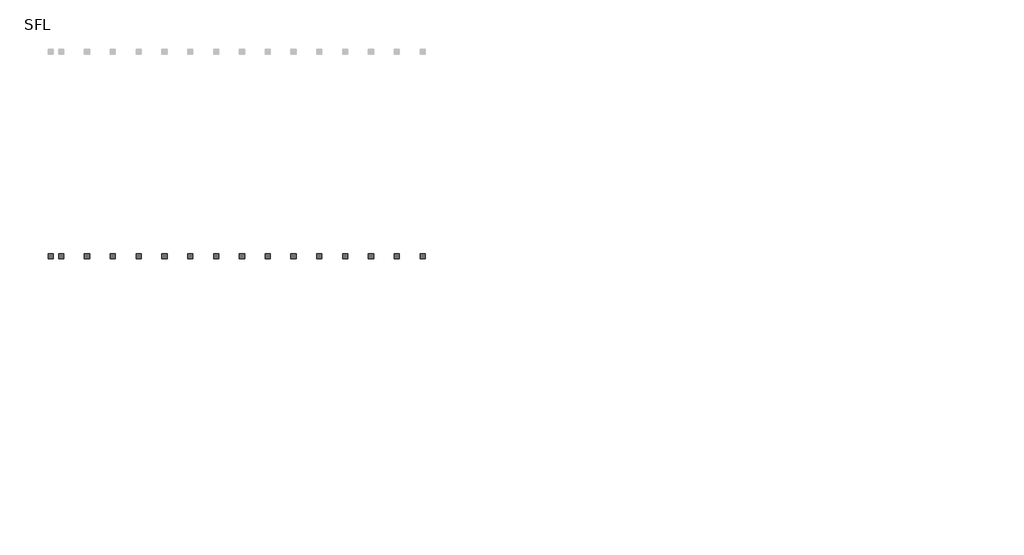
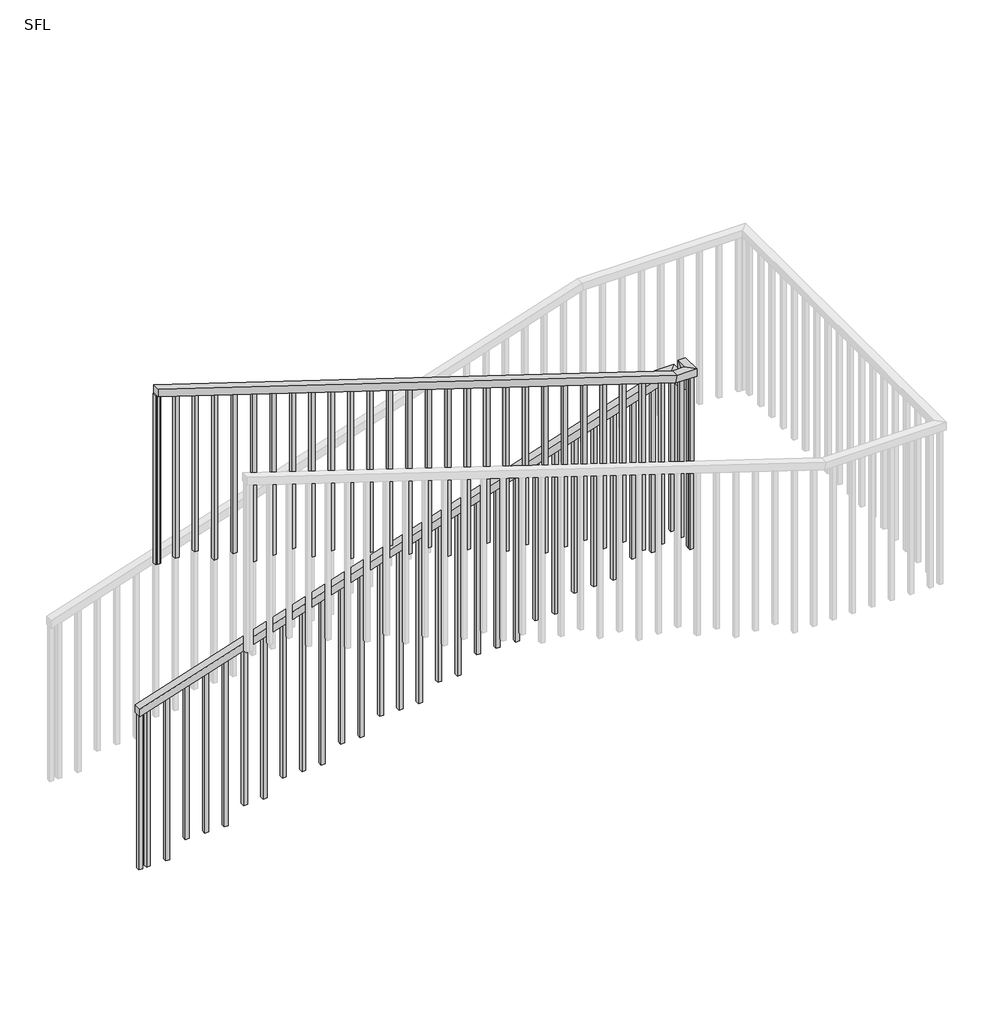
# One storey, part 1 of 2: 1 railing.
"""IFC4 building model written with IfcOpenShell, lengths in millimetres."""

from ifc_helpers import new_model, si_unit, frame, origin, place, context, project, spatial, polyline, outline, extrude, faceted_brep, element, save

model = new_model("IFC4")

# Units and contexts
model_context = context("Model", 3, world=origin())
ifc_project = project(units=[si_unit("LENGTHUNIT", "METRE", prefix="MILLI")], contexts=[model_context])

# Site, building, storey
site = spatial("IfcSite", under=ifc_project)
building = spatial("IfcBuilding", under=site)
storey = spatial("IfcBuildingStorey", under=building, Name="SFL", Elevation=6000.0)

# Railing
placement = place(None, origin())
element("IfcRailing", 1, ObjectType="1100mm", at=placement, inside=storey, context=model_context, shape_type="SolidModel", body=[
    faceted_brep([(-40149.9681829, 16845.7531621, 7799.9767904), (-40149.9681829, 16845.7531621, 7747.4487757), (-40149.9681829, 16795.7531621, 7747.4487757), (-40149.9681829, 16795.7531621, 7799.9767904), (-36808.2681829, 16845.7531621, 8875.9675095), (-36758.2681829, 16845.7531621, 8839.538946), (-36758.2681829, 16795.7531621, 8839.538946), (-36808.2681829, 16795.7531621, 8875.9675095), (-36808.2681829, 16845.7531621, 8899.9878906), (-36758.2681829, 16845.7531621, 8849.9878906), (-36758.2681829, 16795.7531621, 8849.9878906), (-36808.2681829, 16795.7531621, 8899.9878906), (-36683.2681829, 16845.7531621, 8899.9878906), (-36683.2681829, 16845.7531621, 8849.9878906), (-36733.2681829, 16795.7531621, 8849.9878906), (-36733.2681829, 16795.7531621, 8899.9878906), (-36683.2681829, 16720.7531621, 8899.9878906), (-36683.2681829, 16720.7531621, 8849.9878906), (-36733.2681829, 16720.7531621, 8849.9878906), (-36733.2681829, 16720.7531621, 8899.9878906), (-36683.2681829, 16717.5531621, 8899.9878906), (-36683.2681829, 16667.5531621, 8849.9878906), (-36733.2681829, 16667.5531621, 8849.9878906), (-36733.2681829, 16717.5531621, 8899.9878906), (-36683.2681829, 16717.5531621, 9024.0092809), (-36683.2681829, 16667.5531621, 8974.0092809), (-36733.2681829, 16667.5531621, 8974.0092809), (-36733.2681829, 16717.5531621, 9024.0092809), (-36683.2681829, 16592.5531621, 9024.0092809), (-36683.2681829, 16592.5531621, 8974.0092809), (-36733.2681829, 16642.5531621, 8974.0092809), (-36733.2681829, 16642.5531621, 9024.0092809), (-36808.2681829, 16592.5531621, 9024.0092809), (-36816.1194278, 16592.5531621, 8974.0092809), (-36816.1194278, 16642.5531621, 8974.0092809), (-36808.2681829, 16642.5531621, 9024.0092809), (-40149.9681829, 16592.5531621, 10100.0), (-40149.9681829, 16642.5531621, 10100.0), (-40149.9681829, 16642.5531621, 10047.4719853), (-40149.9681829, 16592.5531621, 10047.4719853)], [[[0, 1, 2, 3]], [[1, 0, 4, 5]], [[2, 1, 5, 6]], [[3, 2, 6, 7]], [[0, 3, 7, 4]], [[5, 4, 8, 9]], [[6, 5, 9, 10]], [[7, 6, 10, 11]], [[4, 7, 11, 8]], [[9, 8, 12, 13]], [[10, 9, 13, 14]], [[11, 10, 14, 15]], [[8, 11, 15, 12]], [[13, 12, 16, 17]], [[14, 13, 17, 18]], [[15, 14, 18, 19]], [[12, 15, 19, 16]], [[17, 16, 20, 21]], [[18, 17, 21, 22]], [[19, 18, 22, 23]], [[16, 19, 23, 20]], [[21, 20, 24, 25]], [[22, 21, 25, 26]], [[23, 22, 26, 27]], [[20, 23, 27, 24]], [[25, 24, 28, 29]], [[26, 25, 29, 30]], [[27, 26, 30, 31]], [[24, 27, 31, 28]], [[29, 28, 32, 33]], [[30, 29, 33, 34]], [[31, 30, 34, 35]], [[28, 31, 35, 32]], [[36, 37, 38, 39]], [[33, 32, 36, 39]], [[34, 33, 39, 38]], [[35, 34, 38, 37]], [[32, 35, 37, 36]]]),
    extrude(outline(polyline([(8899.9989909, -40133.2681829), (10042.0947686, -40133.2681829), (10050.1444942, -40158.2681829), (8899.9989909, -40158.2681829), (8899.9989909, -40133.2681829)])), frame((0.0, 16605.0531621, 0.0), z_axis=(0.0, 1.0, 0.0), x_axis=(0.0, 0.0, 1.0)), (0.0, 0.0, 1.0), 25.0),
    extrude(outline(polyline([(8899.9989909, -40008.2681829), (10001.8461407, -40008.2681829), (10009.8958663, -40033.2681829), (8899.9989909, -40033.2681829), (8899.9989909, -40008.2681829)])), frame((0.0, 16605.0531621, 0.0), z_axis=(0.0, 1.0, 0.0), x_axis=(0.0, 0.0, 1.0)), (0.0, 0.0, 1.0), 25.0),
    extrude(outline(polyline([(8899.9989909, -39883.2681829), (9961.5975128, -39883.2681829), (9969.6472384, -39908.2681829), (8899.9989909, -39908.2681829), (8899.9989909, -39883.2681829)])), frame((0.0, 16605.0531621, 0.0), z_axis=(0.0, 1.0, 0.0), x_axis=(0.0, 0.0, 1.0)), (0.0, 0.0, 1.0), 25.0),
    extrude(outline(polyline([(8799.9979818, -39758.2681829), (9921.3488849, -39758.2681829), (9929.3986105, -39783.2681829), (8799.9979818, -39783.2681829), (8799.9979818, -39758.2681829)])), frame((0.0, 16605.0531621, 0.0), z_axis=(0.0, 1.0, 0.0), x_axis=(0.0, 0.0, 1.0)), (0.0, 0.0, 1.0), 25.0),
    extrude(outline(polyline([(8799.9979818, -39633.2681829), (9881.100257, -39633.2681829), (9889.1499826, -39658.2681829), (8799.9979818, -39658.2681829), (8799.9979818, -39633.2681829)])), frame((0.0, 16605.0531621, 0.0), z_axis=(0.0, 1.0, 0.0), x_axis=(0.0, 0.0, 1.0)), (0.0, 0.0, 1.0), 25.0),
    extrude(outline(polyline([(8699.9969727, -39508.2681829), (9840.8516291, -39508.2681829), (9848.9013546, -39533.2681829), (8699.9969727, -39533.2681829), (8699.9969727, -39508.2681829)])), frame((0.0, 16605.0531621, 0.0), z_axis=(0.0, 1.0, 0.0), x_axis=(0.0, 0.0, 1.0)), (0.0, 0.0, 1.0), 25.0),
    extrude(outline(polyline([(8699.9969727, -39383.2681829), (9800.6030011, -39383.2681829), (9808.6527267, -39408.2681829), (8699.9969727, -39408.2681829), (8699.9969727, -39383.2681829)])), frame((0.0, 16605.0531621, 0.0), z_axis=(0.0, 1.0, 0.0), x_axis=(0.0, 0.0, 1.0)), (0.0, 0.0, 1.0), 25.0),
    extrude(outline(polyline([(8699.9969727, -39258.2681829), (9760.3543732, -39258.2681829), (9768.4040988, -39283.2681829), (8699.9969727, -39283.2681829), (8699.9969727, -39258.2681829)])), frame((0.0, 16605.0531621, 0.0), z_axis=(0.0, 1.0, 0.0), x_axis=(0.0, 0.0, 1.0)), (0.0, 0.0, 1.0), 25.0),
    extrude(outline(polyline([(8599.9959635, -39133.2681829), (9720.1057453, -39133.2681829), (9728.1554709, -39158.2681829), (8599.9959635, -39158.2681829), (8599.9959635, -39133.2681829)])), frame((0.0, 16605.0531621, 0.0), z_axis=(0.0, 1.0, 0.0), x_axis=(0.0, 0.0, 1.0)), (0.0, 0.0, 1.0), 25.0),
    extrude(outline(polyline([(8599.9959635, -39008.2681829), (9679.8571174, -39008.2681829), (9687.906843, -39033.2681829), (8599.9959635, -39033.2681829), (8599.9959635, -39008.2681829)])), frame((0.0, 16605.0531621, 0.0), z_axis=(0.0, 1.0, 0.0), x_axis=(0.0, 0.0, 1.0)), (0.0, 0.0, 1.0), 25.0),
    extrude(outline(polyline([(8499.9949544, -38883.2681829), (9639.6084895, -38883.2681829), (9647.6582151, -38908.2681829), (8499.9949544, -38908.2681829), (8499.9949544, -38883.2681829)])), frame((0.0, 16605.0531621, 0.0), z_axis=(0.0, 1.0, 0.0), x_axis=(0.0, 0.0, 1.0)), (0.0, 0.0, 1.0), 25.0),
    extrude(outline(polyline([(8499.9949544, -38758.2681829), (9599.3598616, -38758.2681829), (9607.4095872, -38783.2681829), (8499.9949544, -38783.2681829), (8499.9949544, -38758.2681829)])), frame((0.0, 16605.0531621, 0.0), z_axis=(0.0, 1.0, 0.0), x_axis=(0.0, 0.0, 1.0)), (0.0, 0.0, 1.0), 25.0),
    extrude(outline(polyline([(8499.9949544, -38633.2681829), (9559.1112337, -38633.2681829), (9567.1609593, -38658.2681829), (8499.9949544, -38658.2681829), (8499.9949544, -38633.2681829)])), frame((0.0, 16605.0531621, 0.0), z_axis=(0.0, 1.0, 0.0), x_axis=(0.0, 0.0, 1.0)), (0.0, 0.0, 1.0), 25.0),
    extrude(outline(polyline([(8399.9939453, -38508.2681829), (9518.8626058, -38508.2681829), (9526.9123314, -38533.2681829), (8399.9939453, -38533.2681829), (8399.9939453, -38508.2681829)])), frame((0.0, 16605.0531621, 0.0), z_axis=(0.0, 1.0, 0.0), x_axis=(0.0, 0.0, 1.0)), (0.0, 0.0, 1.0), 25.0),
    extrude(outline(polyline([(8399.9939453, -38383.2681829), (9478.6139779, -38383.2681829), (9486.6637034, -38408.2681829), (8399.9939453, -38408.2681829), (8399.9939453, -38383.2681829)])), frame((0.0, 16605.0531621, 0.0), z_axis=(0.0, 1.0, 0.0), x_axis=(0.0, 0.0, 1.0)), (0.0, 0.0, 1.0), 25.0),
    extrude(outline(polyline([(8299.9929362, -38258.2681829), (9438.36535, -38258.2681829), (9446.4150755, -38283.2681829), (8299.9929362, -38283.2681829), (8299.9929362, -38258.2681829)])), frame((0.0, 16605.0531621, 0.0), z_axis=(0.0, 1.0, 0.0), x_axis=(0.0, 0.0, 1.0)), (0.0, 0.0, 1.0), 25.0),
    extrude(outline(polyline([(8299.9929362, -38133.2681829), (9398.116722, -38133.2681829), (9406.1664476, -38158.2681829), (8299.9929362, -38158.2681829), (8299.9929362, -38133.2681829)])), frame((0.0, 16605.0531621, 0.0), z_axis=(0.0, 1.0, 0.0), x_axis=(0.0, 0.0, 1.0)), (0.0, 0.0, 1.0), 25.0),
    extrude(outline(polyline([(8299.9929362, -38008.2681829), (9357.8680941, -38008.2681829), (9365.9178197, -38033.2681829), (8299.9929362, -38033.2681829), (8299.9929362, -38008.2681829)])), frame((0.0, 16605.0531621, 0.0), z_axis=(0.0, 1.0, 0.0), x_axis=(0.0, 0.0, 1.0)), (0.0, 0.0, 1.0), 25.0),
    extrude(outline(polyline([(8199.9919271, -37883.2681829), (9317.6194662, -37883.2681829), (9325.6691918, -37908.2681829), (8199.9919271, -37908.2681829), (8199.9919271, -37883.2681829)])), frame((0.0, 16605.0531621, 0.0), z_axis=(0.0, 1.0, 0.0), x_axis=(0.0, 0.0, 1.0)), (0.0, 0.0, 1.0), 25.0),
    extrude(outline(polyline([(8199.9919271, -37758.2681829), (9277.3708383, -37758.2681829), (9285.4205639, -37783.2681829), (8199.9919271, -37783.2681829), (8199.9919271, -37758.2681829)])), frame((0.0, 16605.0531621, 0.0), z_axis=(0.0, 1.0, 0.0), x_axis=(0.0, 0.0, 1.0)), (0.0, 0.0, 1.0), 25.0),
    extrude(outline(polyline([(8099.990918, -37633.2681829), (9237.1222104, -37633.2681829), (9245.171936, -37658.2681829), (8099.990918, -37658.2681829), (8099.990918, -37633.2681829)])), frame((0.0, 16605.0531621, 0.0), z_axis=(0.0, 1.0, 0.0), x_axis=(0.0, 0.0, 1.0)), (0.0, 0.0, 1.0), 25.0),
    extrude(outline(polyline([(8099.990918, -37508.2681829), (9196.8735825, -37508.2681829), (9204.9233081, -37533.2681829), (8099.990918, -37533.2681829), (8099.990918, -37508.2681829)])), frame((0.0, 16605.0531621, 0.0), z_axis=(0.0, 1.0, 0.0), x_axis=(0.0, 0.0, 1.0)), (0.0, 0.0, 1.0), 25.0),
    extrude(outline(polyline([(8099.990918, -37383.2681829), (9156.6249546, -37383.2681829), (9164.6746802, -37408.2681829), (8099.990918, -37408.2681829), (8099.990918, -37383.2681829)])), frame((0.0, 16605.0531621, 0.0), z_axis=(0.0, 1.0, 0.0), x_axis=(0.0, 0.0, 1.0)), (0.0, 0.0, 1.0), 25.0),
    extrude(outline(polyline([(7999.9899089, -37258.2681829), (9116.3763267, -37258.2681829), (9124.4260522, -37283.2681829), (7999.9899089, -37283.2681829), (7999.9899089, -37258.2681829)])), frame((0.0, 16605.0531621, 0.0), z_axis=(0.0, 1.0, 0.0), x_axis=(0.0, 0.0, 1.0)), (0.0, 0.0, 1.0), 25.0),
    extrude(outline(polyline([(7999.9899089, -37133.2681829), (9076.1276988, -37133.2681829), (9084.1774243, -37158.2681829), (7999.9899089, -37158.2681829), (7999.9899089, -37133.2681829)])), frame((0.0, 16605.0531621, 0.0), z_axis=(0.0, 1.0, 0.0), x_axis=(0.0, 0.0, 1.0)), (0.0, 0.0, 1.0), 25.0),
    extrude(outline(polyline([(7899.9888997, -37008.2681829), (9035.8790708, -37008.2681829), (9043.9287964, -37033.2681829), (7899.9888997, -37033.2681829), (7899.9888997, -37008.2681829)])), frame((0.0, 16605.0531621, 0.0), z_axis=(0.0, 1.0, 0.0), x_axis=(0.0, 0.0, 1.0)), (0.0, 0.0, 1.0), 25.0),
    extrude(outline(polyline([(7899.9888997, -36883.2681829), (8995.6304429, -36883.2681829), (9003.6801685, -36908.2681829), (7899.9888997, -36908.2681829), (7899.9888997, -36883.2681829)])), frame((0.0, 16605.0531621, 0.0), z_axis=(0.0, 1.0, 0.0), x_axis=(0.0, 0.0, 1.0)), (0.0, 0.0, 1.0), 25.0),
    extrude(outline(polyline([(-36758.2681829, 16630.0531621), (-36758.2681829, 16605.0531621), (-36783.2681829, 16605.0531621), (-36783.2681829, 16630.0531621), (-36758.2681829, 16630.0531621)])), frame((0.0, 0.0, 7899.9888997), z_axis=(0.0, 0.0, 1.0), x_axis=(1.0, 0.0, 0.0)), (0.0, 0.0, 1.0), 1074.0203811),
    extrude(outline(polyline([(-36720.7681829, 16645.7531621), (-36695.7681829, 16645.7531621), (-36695.7681829, 16620.7531621), (-36720.7681829, 16620.7531621), (-36720.7681829, 16645.7531621)])), frame((0.0, 0.0, 7799.9878906), z_axis=(0.0, 0.0, 1.0), x_axis=(1.0, 0.0, 0.0)), (0.0, 0.0, 1.0), 1174.0213903),
    extrude(outline(polyline([(-36720.7681829, 16770.7531621), (-36695.7681829, 16770.7531621), (-36695.7681829, 16745.7531621), (-36720.7681829, 16745.7531621), (-36720.7681829, 16770.7531621)])), frame((0.0, 0.0, 7799.9878906), z_axis=(0.0, 0.0, 1.0), x_axis=(1.0, 0.0, 0.0)), (0.0, 0.0, 1.0), 1050.0),
    extrude(outline(polyline([(-36724.9681829, 16808.2531621), (-36724.9681829, 16833.2531621), (-36699.9681829, 16833.2531621), (-36699.9681829, 16808.2531621), (-36724.9681829, 16808.2531621)])), frame((0.0, 0.0, 7799.9878906), z_axis=(0.0, 0.0, 1.0), x_axis=(1.0, 0.0, 0.0)), (0.0, 0.0, 1.0), 1050.0),
    extrude(outline(polyline([(8810.0125525, -36849.9681829), (7699.9868815, -36849.9681829), (7699.9868815, -36824.9681829), (8818.0622781, -36824.9681829), (8810.0125525, -36849.9681829)])), frame((0.0, 16808.2531621, 0.0), z_axis=(0.0, 1.0, 0.0), x_axis=(0.0, 0.0, 1.0)), (0.0, 0.0, 1.0), 25.0),
    extrude(outline(polyline([(8769.7639246, -36974.9681829), (7699.9868815, -36974.9681829), (7699.9868815, -36949.9681829), (8777.8136502, -36949.9681829), (8769.7639246, -36974.9681829)])), frame((0.0, 16808.2531621, 0.0), z_axis=(0.0, 1.0, 0.0), x_axis=(0.0, 0.0, 1.0)), (0.0, 0.0, 1.0), 25.0),
    extrude(outline(polyline([(8729.5152967, -37099.9681829), (7599.9858724, -37099.9681829), (7599.9858724, -37074.9681829), (8737.5650223, -37074.9681829), (8729.5152967, -37099.9681829)])), frame((0.0, 16808.2531621, 0.0), z_axis=(0.0, 1.0, 0.0), x_axis=(0.0, 0.0, 1.0)), (0.0, 0.0, 1.0), 25.0),
    extrude(outline(polyline([(8689.2666688, -37224.9681829), (7599.9858724, -37224.9681829), (7599.9858724, -37199.9681829), (8697.3163944, -37199.9681829), (8689.2666688, -37224.9681829)])), frame((0.0, 16808.2531621, 0.0), z_axis=(0.0, 1.0, 0.0), x_axis=(0.0, 0.0, 1.0)), (0.0, 0.0, 1.0), 25.0),
    extrude(outline(polyline([(8649.0180409, -37349.9681829), (7599.9858724, -37349.9681829), (7599.9858724, -37324.9681829), (8657.0677665, -37324.9681829), (8649.0180409, -37349.9681829)])), frame((0.0, 16808.2531621, 0.0), z_axis=(0.0, 1.0, 0.0), x_axis=(0.0, 0.0, 1.0)), (0.0, 0.0, 1.0), 25.0),
    extrude(outline(polyline([(8608.769413, -37474.9681829), (7499.9848633, -37474.9681829), (7499.9848633, -37449.9681829), (8616.8191385, -37449.9681829), (8608.769413, -37474.9681829)])), frame((0.0, 16808.2531621, 0.0), z_axis=(0.0, 1.0, 0.0), x_axis=(0.0, 0.0, 1.0)), (0.0, 0.0, 1.0), 25.0),
    extrude(outline(polyline([(8568.5207851, -37599.9681829), (7499.9848633, -37599.9681829), (7499.9848633, -37574.9681829), (8576.5705106, -37574.9681829), (8568.5207851, -37599.9681829)])), frame((0.0, 16808.2531621, 0.0), z_axis=(0.0, 1.0, 0.0), x_axis=(0.0, 0.0, 1.0)), (0.0, 0.0, 1.0), 25.0),
    extrude(outline(polyline([(8528.2721571, -37724.9681829), (7399.9838542, -37724.9681829), (7399.9838542, -37699.9681829), (8536.3218827, -37699.9681829), (8528.2721571, -37724.9681829)])), frame((0.0, 16808.2531621, 0.0), z_axis=(0.0, 1.0, 0.0), x_axis=(0.0, 0.0, 1.0)), (0.0, 0.0, 1.0), 25.0),
    extrude(outline(polyline([(8488.0235292, -37849.9681829), (7399.9838542, -37849.9681829), (7399.9838542, -37824.9681829), (8496.0732548, -37824.9681829), (8488.0235292, -37849.9681829)])), frame((0.0, 16808.2531621, 0.0), z_axis=(0.0, 1.0, 0.0), x_axis=(0.0, 0.0, 1.0)), (0.0, 0.0, 1.0), 25.0),
    extrude(outline(polyline([(8447.7749013, -37974.9681829), (7399.9838542, -37974.9681829), (7399.9838542, -37949.9681829), (8455.8246269, -37949.9681829), (8447.7749013, -37974.9681829)])), frame((0.0, 16808.2531621, 0.0), z_axis=(0.0, 1.0, 0.0), x_axis=(0.0, 0.0, 1.0)), (0.0, 0.0, 1.0), 25.0),
    extrude(outline(polyline([(8407.5262734, -38099.9681829), (7299.9828451, -38099.9681829), (7299.9828451, -38074.9681829), (8415.575999, -38074.9681829), (8407.5262734, -38099.9681829)])), frame((0.0, 16808.2531621, 0.0), z_axis=(0.0, 1.0, 0.0), x_axis=(0.0, 0.0, 1.0)), (0.0, 0.0, 1.0), 25.0),
    extrude(outline(polyline([(8367.2776455, -38224.9681829), (7299.9828451, -38224.9681829), (7299.9828451, -38199.9681829), (8375.3273711, -38199.9681829), (8367.2776455, -38224.9681829)])), frame((0.0, 16808.2531621, 0.0), z_axis=(0.0, 1.0, 0.0), x_axis=(0.0, 0.0, 1.0)), (0.0, 0.0, 1.0), 25.0),
    extrude(outline(polyline([(8327.0290176, -38349.9681829), (7199.9818359, -38349.9681829), (7199.9818359, -38324.9681829), (8335.0787432, -38324.9681829), (8327.0290176, -38349.9681829)])), frame((0.0, 16808.2531621, 0.0), z_axis=(0.0, 1.0, 0.0), x_axis=(0.0, 0.0, 1.0)), (0.0, 0.0, 1.0), 25.0),
    extrude(outline(polyline([(8286.7803897, -38474.9681829), (7199.9818359, -38474.9681829), (7199.9818359, -38449.9681829), (8294.8301153, -38449.9681829), (8286.7803897, -38474.9681829)])), frame((0.0, 16808.2531621, 0.0), z_axis=(0.0, 1.0, 0.0), x_axis=(0.0, 0.0, 1.0)), (0.0, 0.0, 1.0), 25.0),
    extrude(outline(polyline([(8246.5317618, -38599.9681829), (7199.9818359, -38599.9681829), (7199.9818359, -38574.9681829), (8254.5814873, -38574.9681829), (8246.5317618, -38599.9681829)])), frame((0.0, 16808.2531621, 0.0), z_axis=(0.0, 1.0, 0.0), x_axis=(0.0, 0.0, 1.0)), (0.0, 0.0, 1.0), 25.0),
    extrude(outline(polyline([(8206.2831339, -38724.9681829), (7099.9808268, -38724.9681829), (7099.9808268, -38699.9681829), (8214.3328594, -38699.9681829), (8206.2831339, -38724.9681829)])), frame((0.0, 16808.2531621, 0.0), z_axis=(0.0, 1.0, 0.0), x_axis=(0.0, 0.0, 1.0)), (0.0, 0.0, 1.0), 25.0),
    extrude(outline(polyline([(8166.0345059, -38849.9681829), (7099.9808268, -38849.9681829), (7099.9808268, -38824.9681829), (8174.0842315, -38824.9681829), (8166.0345059, -38849.9681829)])), frame((0.0, 16808.2531621, 0.0), z_axis=(0.0, 1.0, 0.0), x_axis=(0.0, 0.0, 1.0)), (0.0, 0.0, 1.0), 25.0),
    extrude(outline(polyline([(8125.785878, -38974.9681829), (6999.9798177, -38974.9681829), (6999.9798177, -38949.9681829), (8133.8356036, -38949.9681829), (8125.785878, -38974.9681829)])), frame((0.0, 16808.2531621, 0.0), z_axis=(0.0, 1.0, 0.0), x_axis=(0.0, 0.0, 1.0)), (0.0, 0.0, 1.0), 25.0),
    extrude(outline(polyline([(8085.5372501, -39099.9681829), (6999.9798177, -39099.9681829), (6999.9798177, -39074.9681829), (8093.5869757, -39074.9681829), (8085.5372501, -39099.9681829)])), frame((0.0, 16808.2531621, 0.0), z_axis=(0.0, 1.0, 0.0), x_axis=(0.0, 0.0, 1.0)), (0.0, 0.0, 1.0), 25.0),
    extrude(outline(polyline([(8045.2886222, -39224.9681829), (6999.9798177, -39224.9681829), (6999.9798177, -39199.9681829), (8053.3383478, -39199.9681829), (8045.2886222, -39224.9681829)])), frame((0.0, 16808.2531621, 0.0), z_axis=(0.0, 1.0, 0.0), x_axis=(0.0, 0.0, 1.0)), (0.0, 0.0, 1.0), 25.0),
    extrude(outline(polyline([(8005.0399943, -39349.9681829), (6899.9788086, -39349.9681829), (6899.9788086, -39324.9681829), (8013.0897199, -39324.9681829), (8005.0399943, -39349.9681829)])), frame((0.0, 16808.2531621, 0.0), z_axis=(0.0, 1.0, 0.0), x_axis=(0.0, 0.0, 1.0)), (0.0, 0.0, 1.0), 25.0),
    extrude(outline(polyline([(7964.7913664, -39474.9681829), (6899.9788086, -39474.9681829), (6899.9788086, -39449.9681829), (7972.841092, -39449.9681829), (7964.7913664, -39474.9681829)])), frame((0.0, 16808.2531621, 0.0), z_axis=(0.0, 1.0, 0.0), x_axis=(0.0, 0.0, 1.0)), (0.0, 0.0, 1.0), 25.0),
    extrude(outline(polyline([(7924.5427385, -39599.9681829), (6799.9777995, -39599.9681829), (6799.9777995, -39574.9681829), (7932.5924641, -39574.9681829), (7924.5427385, -39599.9681829)])), frame((0.0, 16808.2531621, 0.0), z_axis=(0.0, 1.0, 0.0), x_axis=(0.0, 0.0, 1.0)), (0.0, 0.0, 1.0), 25.0),
    extrude(outline(polyline([(7884.2941106, -39724.9681829), (6799.9777995, -39724.9681829), (6799.9777995, -39699.9681829), (7892.3438361, -39699.9681829), (7884.2941106, -39724.9681829)])), frame((0.0, 16808.2531621, 0.0), z_axis=(0.0, 1.0, 0.0), x_axis=(0.0, 0.0, 1.0)), (0.0, 0.0, 1.0), 25.0),
    extrude(outline(polyline([(7844.0454827, -39849.9681829), (6799.9777995, -39849.9681829), (6799.9777995, -39824.9681829), (7852.0952082, -39824.9681829), (7844.0454827, -39849.9681829)])), frame((0.0, 16808.2531621, 0.0), z_axis=(0.0, 1.0, 0.0), x_axis=(0.0, 0.0, 1.0)), (0.0, 0.0, 1.0), 25.0),
    extrude(outline(polyline([(7803.7968547, -39974.9681829), (6699.9767904, -39974.9681829), (6699.9767904, -39949.9681829), (7811.8465803, -39949.9681829), (7803.7968547, -39974.9681829)])), frame((0.0, 16808.2531621, 0.0), z_axis=(0.0, 1.0, 0.0), x_axis=(0.0, 0.0, 1.0)), (0.0, 0.0, 1.0), 25.0),
    extrude(outline(polyline([(7763.5482268, -40099.9681829), (6699.9767904, -40099.9681829), (6699.9767904, -40074.9681829), (7771.5979524, -40074.9681829), (7763.5482268, -40099.9681829)])), frame((0.0, 16808.2531621, 0.0), z_axis=(0.0, 1.0, 0.0), x_axis=(0.0, 0.0, 1.0)), (0.0, 0.0, 1.0), 25.0),
    extrude(outline(polyline([(-36720.7681829, 16630.0531621), (-36695.7681829, 16630.0531621), (-36695.7681829, 16605.0531621), (-36720.7681829, 16605.0531621), (-36720.7681829, 16630.0531621)])), frame((0.0, 0.0, 7799.9878906), z_axis=(0.0, 0.0, 1.0), x_axis=(1.0, 0.0, 0.0)), (0.0, 0.0, 1.0), 1174.0213903),
    extrude(outline(polyline([(-36720.7681829, 16808.2531621), (-36720.7681829, 16833.2531621), (-36695.7681829, 16833.2531621), (-36695.7681829, 16808.2531621), (-36720.7681829, 16808.2531621)])), frame((0.0, 0.0, 7799.9878906), z_axis=(0.0, 0.0, 1.0), x_axis=(1.0, 0.0, 0.0)), (0.0, 0.0, 1.0), 1050.0),
    extrude(outline(polyline([(8899.9989909, -40124.9681829), (10039.4222597, -40124.9681829), (10047.4719853, -40149.9681829), (8899.9989909, -40149.9681829), (8899.9989909, -40124.9681829)])), frame((0.0, 16605.0531621, 0.0), z_axis=(0.0, 1.0, 0.0), x_axis=(0.0, 0.0, 1.0)), (0.0, 0.0, 1.0), 25.0),
    extrude(outline(polyline([(7747.4487757, -40149.9681829), (6699.9767904, -40149.9681829), (6699.9767904, -40124.9681829), (7755.4985013, -40124.9681829), (7747.4487757, -40149.9681829)])), frame((0.0, 16808.2531621, 0.0), z_axis=(0.0, 1.0, 0.0), x_axis=(0.0, 0.0, 1.0)), (0.0, 0.0, 1.0), 25.0),
])

save(model, "model.ifc")

# Revit data of these elements
# Type "1100mm"
#   built-in parameter 1008612 = 0.019685 (stored number, unit not read)
#   built-in parameter 1008611 = 0.019685 (stored number, unit not read)
#   built-in parameter 1008609 = 0.902231 (stored number, unit not read)
#   built-in parameter 1008604 = 0.19685 (stored number, unit not read)
#   built-in parameter 1008603 = 0.164042 (stored number, unit not read)
#   Railing Height = 3' - 7.30709"
#   built-in parameter 1008630 = 2
#   built-in parameter 1008610 = 2
#   built-in parameter 1008608 = 1
#   built-in parameter 1008618 = Baluster_Square : 25mm
# Element 1 (IfcRailing, "1100mm")
#   Phase Created = New Construction
